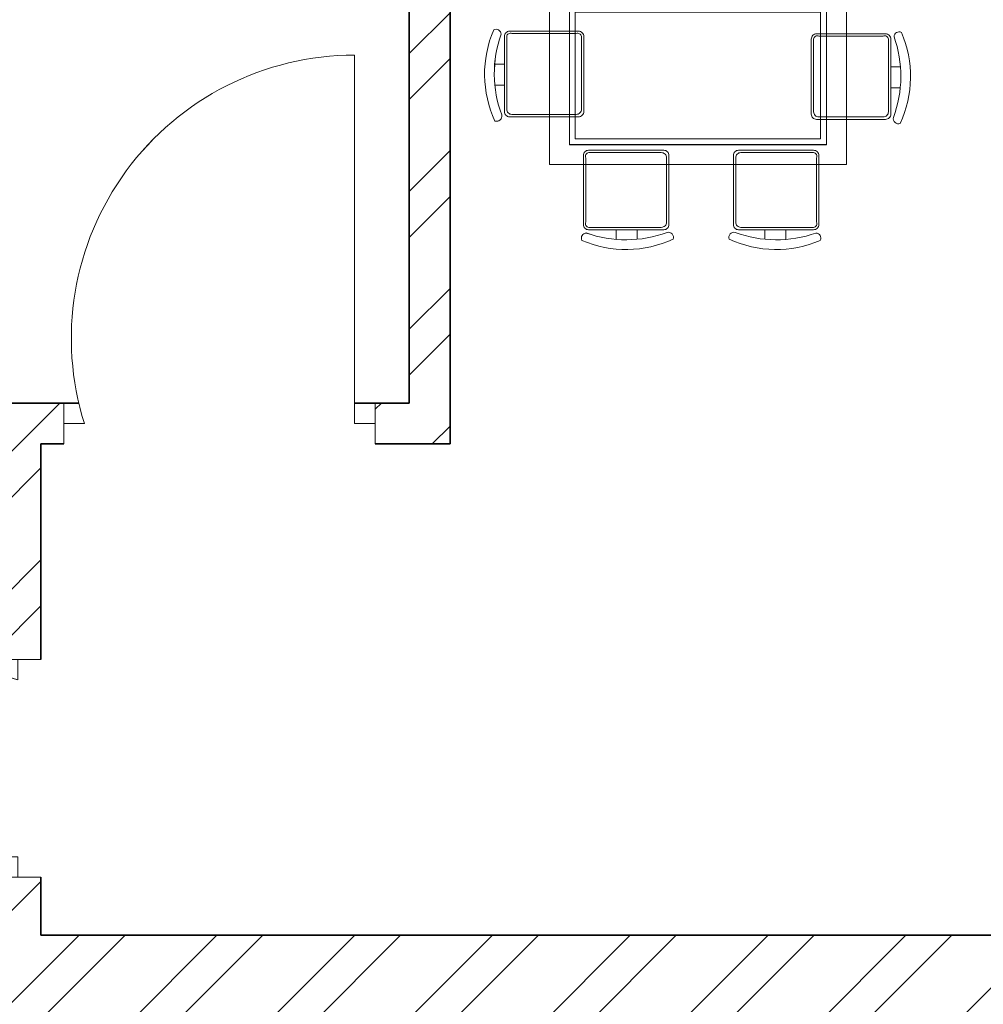
# Model space of a CAD drawing. Units: inches. Extents: x 2120 to 4013, y 1390 to 3019.
# Tile 8 of 59: x 2354 to 2448, y 1868 to 1964. Entities that reach past the tile are written whole.
import ezdxf

# ---------------------------------------------------------------- set-up
doc = ezdxf.new("R2010")
doc.units = ezdxf.units.IN
for name, color, linetype, lineweight in [('A-DOOR', 3, 'Continuous', 18), ('A-FURN', 8, 'Continuous', 13), ('A-WALL', 7, 'Continuous', 35), ('A-WALL-PATT', 252, 'Continuous', 13)]:
    doc.layers.add(name, color=color, linetype=linetype, lineweight=lineweight)

# ---------------------------------------------------------------- blocks, each defined once
blk = doc.blocks.new('DOOR-SWING-24IN-108p49DEG')
for p, q in [((21.75, 21.28), (26.25, 21.28)), ((26.25, 21.28), (24, 21.28)), ((24, 21.28), (24, 19.28)), ((24, 2), (0, 2)), ((24, 0), (24, 2)), ((26.25, 0), (21.75, 0)), ((21.75, 0), (24, 0))]:
    blk.add_line(p, q)
blk.add_arc((18.221, 2), 18.221, 71.50887, 180)
blk = doc.blocks.new('DOOR-SWING-36IN-107p46DEG')
for p, q in [((28.418, 2), (28.418, 38)), ((0, 0), (0, 4)), ((0, 4), (0, 2)), ((30.418, 4), (30.418, 0)), ((0, 2), (2, 2)), ((30.418, 2), (28.418, 2)), ((30.418, 0), (30.418, 2))]:
    blk.add_line(p, q)
blk.add_arc((28.418, 10.307), 27.693, 90, 197.45547)
blk = doc.blocks.new('TABLE-DINING')
for points in [[(0, 17.406), (29.011, 17.406), (29.011, 0), (0, 0)], [(1.934, 15.472), (27.077, 15.472), (27.077, 1.934), (1.934, 1.934)], [(2.514, 14.892), (26.496, 14.892), (26.496, 2.514), (2.514, 2.514)]]:
    blk.add_lwpolyline(points, close=True)
blk = doc.blocks.new('CHAIR-DINING-04')
for points in [[(7.771, 8.294, 0.414214), (7.258, 8.807), (0.513, 8.807, 0.414214), (0, 8.294), (0, 0.958, 0.414214), (0.513, 0.445), (7.258, 0.445, 0.414214), (7.771, 0.958), (7.771, 8.294)], [(8.089, 8.525, -0.175809), (8.029, 0.623, 0.578392), (8.687, 0.025, 0.214524), (8.807, 8.944, 0.552014), (8.089, 8.525, -0.065079)], [(7.771, 3.535), (8.699, 3.535, -0.064759)]]:
    blk.add_lwpolyline(points, format="xyb")
blk.add_lwpolyline([(7.54, 8.291), (7.54, 1.19, -0.414214), (7.027, 0.676), (0.744, 0.676, -0.414214), (0.231, 1.19), (0.231, 8.291, -0.512069), (0.744, 8.576), (7.027, 8.576, -0.512069)], format="xyb", close=True)
blk.add_lwpolyline([(8.716, 5.588), (7.771, 5.588)])
blk = doc.blocks.new('CHAIR-DINING-05')
for points in [[(1.676, 0.623, -0.578392), (1.018, 0.025, -0.214524), (0.898, 8.944, -0.552014), (1.616, 8.525, 0.175809), (1.676, 0.623)], [(1.933, 8.294, -0.414214), (2.446, 8.807), (9.191, 8.807, -0.414214), (9.704, 8.294), (9.704, 0.958, -0.414214), (9.191, 0.445), (2.446, 0.445, -0.414214), (1.933, 0.958), (1.933, 8.294)], [(1.933, 3.535), (1.005, 3.535, 0.064759)]]:
    blk.add_lwpolyline(points, format="xyb")
blk.add_lwpolyline([(2.164, 8.291), (2.164, 1.19, 0.414214), (2.677, 0.676), (8.96, 0.676, 0.414214), (9.473, 1.19), (9.473, 8.291, 0.512069), (8.96, 8.576), (2.677, 8.576, 0.512069)], format="xyb", close=True)
blk.add_lwpolyline([(0.988, 5.588), (1.933, 5.588)])
blk = doc.blocks.new('CHAIR-DINING-10')
for points in [[(0.623, 8.029, -0.578392), (0.025, 8.687, -0.214524), (8.944, 8.807, -0.552014), (8.525, 8.089, 0.175809), (0.623, 8.029)], [(3.535, 7.771), (3.535, 8.699, 0.064759)], [(8.294, 7.771, -0.414214), (8.807, 7.258), (8.807, 0.513, -0.414214), (8.294, 0), (0.958, 0, -0.414214), (0.445, 0.513), (0.445, 7.258, -0.414214), (0.958, 7.771), (8.294, 7.771)]]:
    blk.add_lwpolyline(points, format="xyb")
blk.add_lwpolyline([(5.588, 8.716), (5.588, 7.771)])
blk.add_lwpolyline([(8.291, 7.54), (1.19, 7.54, 0.414214), (0.676, 7.027), (0.676, 0.744, 0.414214), (1.19, 0.231), (8.291, 0.231, 0.512069), (8.576, 0.744), (8.576, 7.027, 0.512069)], format="xyb", close=True)
blk = doc.blocks.new('CHAIR-DINING-15')
for points in [[(8.294, 1.933, 0.414214), (8.807, 2.446), (8.807, 9.191, 0.414214), (8.294, 9.704), (0.958, 9.704, 0.414214), (0.445, 9.191), (0.445, 2.446, 0.414214), (0.958, 1.933), (8.294, 1.933)], [(3.535, 1.933), (3.535, 1.005, -0.064759)], [(8.525, 1.616, -0.175809), (0.623, 1.676, 0.578392), (0.025, 1.018, 0.214524), (8.944, 0.898, 0.552014), (8.525, 1.616, -0.065079)]]:
    blk.add_lwpolyline(points, format="xyb")
blk.add_lwpolyline([(8.291, 2.164), (1.19, 2.164, -0.414214), (0.676, 2.677), (0.676, 8.96, -0.414214), (1.19, 9.473), (8.291, 9.473, -0.512069), (8.576, 8.96), (8.576, 2.677, -0.512069)], format="xyb", close=True)
blk.add_lwpolyline([(5.588, 0.988), (5.588, 1.933)])

msp = doc.modelspace()

# ---------------------------------------------------------------- hatches: boundary and pattern name
at = {"layer": 'A-WALL-PATT'}
h = msp.add_hatch(dxfattribs=at)
h.set_pattern_fill('ANSI32', color=256)
h.paths.add_polyline_path([(2271.7331, 1980.389), (2262.7331, 1980.389), (2262.7331, 1912.8434), (2267.2331, 1912.8434), (2271.7331, 1912.8434), (2271.7331, 1922.531), (2351.2331, 1922.531), (2351.2331, 1901.4728), (2355.7331, 1901.4728), (2355.7331, 1922.531), (2357.9815, 1922.531), (2357.9815, 1926.5306), (2271.7331, 1926.5306)])
h.paths.add_polyline_path([(2589.2331, 1949.1622), (2584.7331, 1949.1622), (2580.2331, 1949.1622), (2580.2331, 1874.5306), (2355.7331, 1874.5306), (2355.7331, 1880.1922), (2351.2331, 1880.1922), (2351.2331, 1874.5306), (2271.7331, 1874.5306), (2271.7331, 1888.8431), (2262.7331, 1888.8431), (2262.7331, 1842.2909), (2267.2331, 1842.2909), (2271.7331, 1842.2909), (2271.7331, 1865.531), (2415.7331, 1865.531), (2415.7331, 1779.7286), (2420.2331, 1779.7286), (2420.2331, 1865.531), (2589.2331, 1865.531)])
h.paths.add_polyline_path([(2271.7331, 1782.2906), (2262.7331, 1782.2906), (2262.7331, 1711.4639), (2267.2331, 1711.4639), (2271.7331, 1711.4639), (2271.7331, 1738.031), (2420.2331, 1738.031), (2420.2331, 1742.531), (2420.2331, 1747.3376), (2417.9831, 1747.3376), (2415.7331, 1747.3376), (2415.7331, 1742.5306), (2271.7331, 1742.5306)])
h.paths.add_polyline_path([(2271.7331, 1627.031), (2362.3957, 1627.031), (2362.3957, 1629.281), (2362.3957, 1631.5306), (2271.7331, 1631.5306), (2271.7331, 1675.4636), (2262.7331, 1675.4636), (2262.7331, 1581.531), (2405.3032, 1581.531), (2405.3032, 1586.031), (2405.3032, 1590.5306), (2396.2331, 1590.5306), (2396.2331, 1691.4513), (2418.7206, 1691.4513), (2418.7206, 1695.951), (2396.2331, 1695.951), (2391.7331, 1695.951), (2391.7331, 1631.5306), (2386.7425, 1631.5306), (2386.7425, 1629.2806), (2386.7425, 1627.031), (2391.7331, 1627.031), (2391.7331, 1586.1709), (2271.7331, 1586.1709)])
h.paths.add_polyline_path([(2459.6703, 1590.5306), (2429.3032, 1590.5306), (2429.3032, 1581.531), (2459.6703, 1581.531), (2459.6703, 1586.031)])
h.paths.add_polyline_path([(2501.2331, 1590.531), (2501.2331, 1665.0195), (2498.9831, 1665.0195), (2496.7331, 1665.0195), (2496.7331, 1590.5306), (2483.8201, 1590.5306), (2483.8201, 1590.1579), (2483.6704, 1590.1579), (2483.6704, 1581.531), (2505.0196, 1581.531), (2505.0196, 1583.781), (2505.0196, 1586.0306), (2501.2331, 1586.0306)])
h.paths.add_polyline_path([(2544.1361, 1583.781), (2544.1361, 1586.0306), (2527.1368, 1586.0306), (2527.1368, 1583.7806), (2527.1368, 1581.531), (2544.1361, 1581.531)])
h.paths.add_polyline_path([(3822.6535, 2458.4402), (3874.9468, 2458.4402), (3874.9468, 2476.9866), (3822.6535, 2476.9866)], flags=9)
h.paths.add_polyline_path([(3834.6921, 2781.8174), (3935.9206, 2781.8174), (3935.9206, 2800.3638), (3834.6921, 2800.3638)], flags=9)
h.paths.add_polyline_path([(3832.2843, 2837.9683), (3884.5776, 2837.9683), (3884.5776, 2856.5146), (3832.2843, 2856.5146)], flags=9)
h.paths.add_polyline_path([(3830.9388, 2861.4782), (3956.8958, 2861.4782), (3956.8958, 2880.0245), (3830.9388, 2880.0245)], flags=9)
h.paths.add_polyline_path([(3870.6966, 2352.5752), (3887.9272, 2352.5752), (3887.9272, 2377.3037), (3870.6966, 2377.3037)], flags=9)
h.paths.add_polyline_path([(3289.2701, 2413.161), (3435.2223, 2413.161), (3435.2223, 2450.2538), (3289.2701, 2450.2538)], flags=9)
h.paths.add_polyline_path([(2487.6944, 2414.3601), (2637.8335, 2414.3601), (2637.8335, 2451.4528), (2487.6944, 2451.4528)], flags=9)
h.paths.add_polyline_path([(2567.3724, 1457.9199), (2815.296, 1457.9199), (2815.296, 1495.0127), (2567.3724, 1495.0127)], flags=9)
h.paths.add_polyline_path([(2655.3825, 2093.2363), (2685.9555, 2093.2363), (2685.9555, 2111.8937), (2655.3825, 2111.8937)], flags=9)
h.paths.add_polyline_path([(2543.9218, 1550.6671), (2587.8406, 1550.6671), (2587.8406, 1569.3244), (2543.9218, 1569.3244)], flags=9)
h.paths.add_polyline_path([(2905.1384, 1543.8113), (2949.0572, 1543.8113), (2949.0572, 1562.4686), (2905.1384, 1562.4686)], flags=9)
h.paths.add_polyline_path([(2736.4118, 1702.4736), (2784.2153, 1702.4736), (2784.2153, 1721.1309), (2736.4118, 1721.1309)], flags=9)
h.paths.add_polyline_path([(2912.8666, 1710.4168), (2951.707, 1710.4168), (2951.707, 1729.0741), (2912.8666, 1729.0741)], flags=9)
h.paths.add_polyline_path([(2923.5785, 1763.5038), (2959.7279, 1763.5038), (2959.7279, 1782.1611), (2923.5785, 1782.1611)], flags=9)
h.paths.add_polyline_path([(2925.2114, 1809.6137), (2967.1861, 1809.6137), (2967.1861, 1828.271), (2925.2114, 1828.271)], flags=9)
h.paths.add_polyline_path([(2996.2711, 1878.9003), (2996.2711, 1913.109), (2977.6138, 1913.109), (2977.6138, 1878.9003)], flags=9)
h.paths.add_polyline_path([(2883.0859, 1895.7192), (2927.1855, 1895.7192), (2927.1855, 1914.3766), (2883.0859, 1914.3766)], flags=9)
h.paths.add_polyline_path([(2787.3924, 1810.8013), (2841.0213, 1810.8013), (2841.0213, 1829.4587), (2787.3924, 1829.4587)], flags=9)
h.paths.add_polyline_path([(2775.6399, 2101.7395), (2829.2689, 2101.7395), (2829.2689, 2120.3968), (2775.6399, 2120.3968)], flags=9)
h.paths.add_polyline_path([(2913.0263, 2075.817), (2951.8667, 2075.817), (2951.8667, 2094.4744), (2913.0263, 2094.4744)], flags=9)
h.paths.add_polyline_path([(2929.966, 2133.3669), (2966.1154, 2133.3669), (2966.1154, 2152.0243), (2929.966, 2152.0243)], flags=9)
h.paths.add_polyline_path([(2932.7502, 2182.6088), (2968.8996, 2182.6088), (2968.8996, 2201.2662), (2932.7502, 2201.2662)], flags=9)
h.paths.add_polyline_path([(2996.0681, 2266.3173), (2996.0681, 2300.5261), (2977.4108, 2300.5261), (2977.4108, 2266.3173)], flags=9)
h.paths.add_polyline_path([(2885.1039, 2279.2186), (2929.2035, 2279.2186), (2929.2035, 2297.8759), (2885.1039, 2297.8759)], flags=9)
h.paths.add_polyline_path([(2735.7042, 2218.3197), (2783.5078, 2218.3197), (2783.5078, 2236.9771), (2735.7042, 2236.9771)], flags=9)
h.paths.add_polyline_path([(2635.6049, 2044.0085), (2648.9678, 2044.0085), (2648.9678, 2054.312), (2635.6049, 2054.312)], flags=9)
h.paths.add_polyline_path([(2714.0148, 1923.0473), (2727.3777, 1923.0473), (2727.3777, 1933.3508), (2714.0148, 1933.3508)], flags=9)
h.paths.add_polyline_path([(2709.0345, 1988.1628), (2722.3974, 1988.1628), (2722.3974, 1998.4663), (2709.0345, 1998.4663)], flags=9)
h.paths.add_polyline_path([(2592.8935, 1962.1763), (2606.2564, 1962.1763), (2606.2564, 1972.4799), (2592.8935, 1972.4799)], flags=9)
h.paths.add_polyline_path([(2618.3996, 1985.9724), (2644.1942, 1985.9724), (2644.1942, 1996.2759), (2618.3996, 1996.2759)], flags=9)
h.paths.add_polyline_path([(2601.279, 1920.5869), (2614.6419, 1920.5869), (2614.6419, 1930.8904), (2601.279, 1930.8904)], flags=9)
h.paths.add_polyline_path([(2692.3278, 1932.7645), (2704.5311, 1932.7645), (2704.5311, 1943.0681), (2692.3278, 1943.0681)], flags=9)
h.paths.add_polyline_path([(2311.122, 1672.7318), (2355.0408, 1672.7318), (2355.0408, 1691.3892), (2311.122, 1691.3892)], flags=25)
h.paths.add_polyline_path([(2456.2551, 1632.3198), (2492.4796, 1632.3198), (2492.4796, 1650.9772), (2456.2551, 1650.9772)], flags=9)
h.paths.add_polyline_path([(2401.0766, 1631.4793), (2437.301, 1631.4793), (2437.301, 1650.1367), (2401.0766, 1650.1367)], flags=9)
h.paths.add_polyline_path([(2546.7054, 1700.9235), (2594.509, 1700.9235), (2594.509, 1719.5809), (2546.7054, 1719.5809)], flags=9)
h.paths.add_polyline_path([(2445.4866, 1766.9937), (2497.5261, 1766.9937), (2497.5261, 1785.651), (2445.4866, 1785.651)], flags=9)
h.paths.add_polyline_path([(2287.9992, 1739.7675), (2326.8396, 1739.7675), (2326.8396, 1758.4248), (2287.9992, 1758.4248)], flags=24)
h.paths.add_polyline_path([(2458.5279, 1924.7607), (2510.5675, 1924.7607), (2510.5675, 1943.4181), (2458.5279, 1943.4181)], flags=25)
h.paths.add_polyline_path([(2309.2811, 1902.7642), (2345.4305, 1902.7642), (2345.4305, 1921.4215), (2309.2811, 1921.4215)], flags=25)
h.paths.add_polyline_path([(2490.7554, 2018.9392), (2530.7896, 2018.9392), (2530.7896, 2037.5965), (2490.7554, 2037.5965)], flags=9)
h.paths.add_polyline_path([(2402.143, 2024.7393), (2438.5414, 2024.7393), (2438.5414, 2043.3966), (2402.143, 2043.3966)], flags=9)
h.paths.add_polyline_path([(2287.856, 1931.7926), (2326.6964, 1931.7926), (2326.6964, 1950.4499), (2287.856, 1950.4499)], flags=25)
h.paths.add_polyline_path([(2281.7979, 2193.5771), (2320.6383, 2193.5771), (2320.6383, 2212.2344), (2281.7979, 2212.2344)], flags=9)
h.paths.add_polyline_path([(2484.0754, 2093.892), (2536.115, 2093.892), (2536.115, 2112.5494), (2484.0754, 2112.5494)], flags=9)
h.paths.add_polyline_path([(2624.7948, 2281.8639), (2624.7948, 2311.4137), (2606.1375, 2311.4137), (2606.1375, 2281.8639)], flags=9)
h.paths.add_polyline_path([(2507.5036, 2290.3639), (2541.934, 2290.3639), (2541.934, 2309.0212), (2507.5036, 2309.0212)], flags=9)
h.paths.add_polyline_path([(2423.1076, 2285.2202), (2459.332, 2285.2202), (2459.332, 2303.8776), (2423.1076, 2303.8776)], flags=9)
h.paths.add_polyline_path([(2374.5467, 2289.6272), (2410.7711, 2289.6272), (2410.7711, 2308.2846), (2374.5467, 2308.2846)], flags=9)
h.paths.add_polyline_path([(2277.4907, 2227.5651), (2316.3311, 2227.5651), (2316.3311, 2246.2224), (2277.4907, 2246.2224)], flags=9)
h.paths.add_polyline_path([(2655.3825, 2093.2367), (2685.9555, 2093.2367), (2685.9555, 2111.894), (2655.3825, 2111.894)], flags=9)
h.paths.add_polyline_path([(2543.9217, 1550.6674), (2587.8406, 1550.6674), (2587.8406, 1569.3247), (2543.9217, 1569.3247)], flags=9)
h.paths.add_polyline_path([(2905.1384, 1543.8116), (2949.0572, 1543.8116), (2949.0572, 1562.4689), (2905.1384, 1562.4689)], flags=9)
h.paths.add_polyline_path([(2736.4118, 1702.4739), (2784.2153, 1702.4739), (2784.2153, 1721.1312), (2736.4118, 1721.1312)], flags=9)
h.paths.add_polyline_path([(2912.8666, 1710.4171), (2951.707, 1710.4171), (2951.707, 1729.0744), (2912.8666, 1729.0744)], flags=9)
h.paths.add_polyline_path([(2923.5785, 1763.5041), (2959.7279, 1763.5041), (2959.7279, 1782.1614), (2923.5785, 1782.1614)], flags=9)
h.paths.add_polyline_path([(2925.2114, 1809.614), (2967.1861, 1809.614), (2967.1861, 1828.2713), (2925.2114, 1828.2713)], flags=9)
h.paths.add_polyline_path([(2996.2711, 1878.9006), (2996.2711, 1913.1094), (2977.6137, 1913.1094), (2977.6137, 1878.9006)], flags=9)
h.paths.add_polyline_path([(2883.0859, 1895.7195), (2927.1855, 1895.7195), (2927.1855, 1914.3769), (2883.0859, 1914.3769)], flags=9)
h.paths.add_polyline_path([(2787.3924, 1810.8016), (2841.0213, 1810.8016), (2841.0213, 1829.459), (2787.3924, 1829.459)], flags=9)
h.paths.add_polyline_path([(2775.6399, 2101.7398), (2829.2688, 2101.7398), (2829.2688, 2120.3971), (2775.6399, 2120.3971)], flags=9)
h.paths.add_polyline_path([(2913.0263, 2075.8173), (2951.8667, 2075.8173), (2951.8667, 2094.4747), (2913.0263, 2094.4747)], flags=9)
h.paths.add_polyline_path([(2929.966, 2133.3672), (2966.1154, 2133.3672), (2966.1154, 2152.0246), (2929.966, 2152.0246)], flags=9)
h.paths.add_polyline_path([(2932.7502, 2182.6091), (2968.8996, 2182.6091), (2968.8996, 2201.2665), (2932.7502, 2201.2665)], flags=9)
h.paths.add_polyline_path([(2996.0681, 2266.3176), (2996.0681, 2300.5264), (2977.4108, 2300.5264), (2977.4108, 2266.3176)], flags=9)
h.paths.add_polyline_path([(2885.1039, 2279.2189), (2929.2035, 2279.2189), (2929.2035, 2297.8762), (2885.1039, 2297.8762)], flags=9)
h.paths.add_polyline_path([(2735.7042, 2218.32), (2783.5078, 2218.32), (2783.5078, 2236.9774), (2735.7042, 2236.9774)], flags=9)
h.paths.add_polyline_path([(2635.6048, 2044.0088), (2648.9677, 2044.0088), (2648.9677, 2054.3123), (2635.6048, 2054.3123)], flags=9)
h.paths.add_polyline_path([(2714.0148, 1923.0476), (2727.3777, 1923.0476), (2727.3777, 1933.3511), (2714.0148, 1933.3511)], flags=9)
h.paths.add_polyline_path([(2709.0345, 1988.1631), (2722.3974, 1988.1631), (2722.3974, 1998.4666), (2709.0345, 1998.4666)], flags=9)
h.paths.add_polyline_path([(2592.8935, 1962.1766), (2606.2564, 1962.1766), (2606.2564, 1972.4802), (2592.8935, 1972.4802)], flags=9)
h.paths.add_polyline_path([(2618.3995, 1985.9727), (2644.1942, 1985.9727), (2644.1942, 1996.2762), (2618.3995, 1996.2762)], flags=9)
h.paths.add_polyline_path([(2601.279, 1920.5872), (2614.6419, 1920.5872), (2614.6419, 1930.8908), (2601.279, 1930.8908)], flags=9)
h.paths.add_polyline_path([(2692.3278, 1932.7648), (2704.5311, 1932.7648), (2704.5311, 1943.0684), (2692.3278, 1943.0684)], flags=9)
h.paths.add_polyline_path([(2311.122, 1672.7321), (2355.0408, 1672.7321), (2355.0408, 1691.3895), (2311.122, 1691.3895)], flags=25)
h.paths.add_polyline_path([(2456.2551, 1632.3201), (2492.4795, 1632.3201), (2492.4795, 1650.9775), (2456.2551, 1650.9775)], flags=9)
h.paths.add_polyline_path([(2401.0766, 1631.4796), (2437.301, 1631.4796), (2437.301, 1650.137), (2401.0766, 1650.137)], flags=9)
h.paths.add_polyline_path([(2546.7054, 1700.9238), (2594.509, 1700.9238), (2594.509, 1719.5812), (2546.7054, 1719.5812)], flags=9)
h.paths.add_polyline_path([(2445.4866, 1766.994), (2497.5261, 1766.994), (2497.5261, 1785.6513), (2445.4866, 1785.6513)], flags=9)
h.paths.add_polyline_path([(2287.9992, 1739.7678), (2326.8396, 1739.7678), (2326.8396, 1758.4251), (2287.9992, 1758.4251)], flags=24)
h.paths.add_polyline_path([(2458.5279, 1924.7611), (2510.5675, 1924.7611), (2510.5675, 1943.4184), (2458.5279, 1943.4184)], flags=25)
h.paths.add_polyline_path([(2309.2811, 1902.7645), (2345.4305, 1902.7645), (2345.4305, 1921.4218), (2309.2811, 1921.4218)], flags=25)
h.paths.add_polyline_path([(2490.7554, 2018.9395), (2530.7895, 2018.9395), (2530.7895, 2037.5968), (2490.7554, 2037.5968)], flags=9)
h.paths.add_polyline_path([(2402.143, 2024.7396), (2438.5413, 2024.7396), (2438.5413, 2043.3969), (2402.143, 2043.3969)], flags=9)
h.paths.add_polyline_path([(2287.856, 1931.7929), (2326.6964, 1931.7929), (2326.6964, 1950.4502), (2287.856, 1950.4502)], flags=25)
h.paths.add_polyline_path([(2281.7979, 2193.5774), (2320.6383, 2193.5774), (2320.6383, 2212.2347), (2281.7979, 2212.2347)], flags=9)
h.paths.add_polyline_path([(2484.0754, 2093.8924), (2536.115, 2093.8924), (2536.115, 2112.5497), (2484.0754, 2112.5497)], flags=9)
h.paths.add_polyline_path([(2624.7948, 2281.8642), (2624.7948, 2311.414), (2606.1374, 2311.414), (2606.1374, 2281.8642)], flags=9)
h.paths.add_polyline_path([(2507.5035, 2290.3642), (2541.934, 2290.3642), (2541.934, 2309.0215), (2507.5035, 2309.0215)], flags=9)
h.paths.add_polyline_path([(2423.1075, 2285.2205), (2459.332, 2285.2205), (2459.332, 2303.8779), (2423.1075, 2303.8779)], flags=9)
h.paths.add_polyline_path([(2374.5467, 2289.6275), (2410.7711, 2289.6275), (2410.7711, 2308.2849), (2374.5467, 2308.2849)], flags=9)
h.paths.add_polyline_path([(2277.4907, 2227.5654), (2316.3311, 2227.5654), (2316.3311, 2246.2227), (2277.4907, 2246.2227)], flags=9)
h = msp.add_hatch(dxfattribs=at)
h.set_pattern_fill('ANSI32', color=256)
h.paths.add_polyline_path([(2271.7331, 2122.6377), (2262.7331, 2122.6377), (2262.7331, 2040.3893), (2267.2331, 2040.3893), (2271.7331, 2040.3893), (2271.7331, 2044.8856), (2271.7331, 2070.531), (2391.7331, 2070.531), (2391.7331, 1926.5306), (2388.3993, 1926.5306), (2388.3993, 1922.531), (2395.7331, 1922.531), (2395.7331, 1992.531), (2400.4511, 1992.531), (2400.4511, 1997.0306), (2395.7331, 1997.0306), (2395.7331, 2070.531), (2443.7331, 2070.531), (2443.7331, 2046.1368), (2448.2331, 2046.1368), (2448.2331, 2070.531), (2580.2331, 2070.531), (2580.2331, 1997.0306), (2492.9076, 1997.0306), (2492.9076, 1992.531), (2580.2331, 1992.531), (2580.2331, 1983.9368), (2589.2331, 1983.9368), (2589.2331, 2070.531), (2589.2331, 2075.0306), (2396.2331, 2075.0306), (2396.2331, 2184.3565), (2393.9831, 2184.3565), (2391.7331, 2184.3565), (2391.7331, 2075.0306), (2271.7331, 2075.0306)])
h.paths.add_polyline_path([(2724.7331, 2138.0306), (2628.7331, 2138.0306), (2628.7331, 2070.5306), (2628.7331, 2067.0987), (2633.2331, 2067.0987), (2637.7331, 2067.0987), (2637.7331, 2070.531), (2657.3413, 2070.531), (2657.3413, 2079.5306), (2637.7331, 2079.5306), (2637.7331, 2129.031), (2715.7331, 2129.031), (2715.7331, 2079.5306), (2698.0378, 2079.5306), (2698.0378, 2070.531), (2715.7331, 2070.531), (2715.7331, 2012.1531), (2720.2331, 2012.1531), (2724.7331, 2012.1531)])
h.paths.add_polyline_path([(2724.7331, 2213.031), (2831.3209, 2213.031), (2831.3209, 2215.281), (2831.3209, 2217.5306), (2724.7331, 2217.5306), (2724.7331, 2343.531), (2751.8755, 2343.531), (2751.8755, 2352.5306), (2715.7331, 2352.5306), (2715.7331, 2138.031), (2724.7331, 2138.031)])
h.paths.add_polyline_path([(2902.53, 2352.5306), (2811.8755, 2352.5306), (2811.8755, 2343.531), (2867.2331, 2343.531), (2867.2331, 2217.5306), (2863.6364, 2217.5306), (2863.6364, 2213.031), (2871.7331, 2213.031), (2871.7331, 2217.531), (2871.7331, 2343.531), (2902.53, 2343.531)])
h.paths.add_polyline_path([(3009.7331, 2352.5306), (2938.53, 2352.5306), (2938.53, 2343.531), (2966.2331, 2343.531), (2966.2331, 2242.3281), (2968.4831, 2242.3281), (2970.7331, 2242.3281), (2970.7331, 2343.531), (3009.7331, 2343.531)])
h.paths.add_polyline_path([(3009.7331, 2217.5306), (2970.7331, 2217.5306), (2970.7331, 2220.5422), (2968.4831, 2220.5422), (2966.2331, 2220.5422), (2966.2331, 2217.5306), (2911.7752, 2217.5306), (2907.7331, 2217.5306), (2907.7331, 2213.0306), (2907.7331, 2194.9663), (2912.2331, 2194.9663), (2912.2331, 2213.031), (2970.7331, 2213.031), (3000.7331, 2213.031), (3000.7331, 2205.523), (3009.7331, 2205.523)])
h.paths.add_polyline_path([(3009.7331, 2181.5227), (3000.7331, 2181.5227), (3000.7331, 2165.0306), (2912.2331, 2165.0306), (2912.2331, 2170.8202), (2907.7331, 2170.8202), (2907.7331, 2165.0306), (2899.5169, 2165.0306), (2899.5169, 2162.7806), (2899.5169, 2160.531), (2907.7331, 2160.531), (2907.7331, 2137.3432), (2912.2331, 2137.3432), (2912.2331, 2160.531), (3000.7331, 2160.531), (3000.7331, 2150.4993), (3009.7331, 2150.4993)])
h.paths.add_polyline_path([(3009.7331, 2126.499), (3005.2331, 2126.499), (3000.7331, 2126.499), (3000.7331, 2112.5306), (2912.2331, 2112.5306), (2912.2331, 2115.6036), (2907.7331, 2115.6036), (2907.7331, 2108.031), (3000.7331, 2108.031), (3000.7331, 2084.7256), (3009.7331, 2084.7256)], flags=17)
h.paths.add_polyline_path([(3009.7331, 1971.531), (3009.7331, 2024.7253), (3000.7331, 2024.7253), (3000.7331, 2006.4153), (3000.7331, 1971.5306), (2864.2331, 1971.5306), (2864.2331, 2160.531), (2868.0522, 2160.531), (2868.0522, 2165.0306), (2859.7331, 2165.0306), (2859.7331, 1971.5306), (2724.7331, 1971.5306), (2724.7331, 1977.7012), (2715.7331, 1977.7012), (2715.7331, 1962.5306), (2715.7331, 1950.9035), (2720.2331, 1950.9035), (2724.7331, 1950.9035), (2724.7331, 1962.531), (2855.2331, 1962.531), (2859.7331, 1962.531), (2859.7331, 1835.031), (2864.2331, 1834.8158), (2864.2331, 1962.531), (2958.7331, 1962.531), (2958.7331, 1937.0925), (2963.2331, 1937.0925), (2963.2331, 1962.531), (3000.7331, 1962.531), (3009.7331, 1962.531)])
h.paths.add_polyline_path([(2724.7331, 1728.531), (2822.7164, 1728.531), (2822.7164, 1733.0306), (2724.7331, 1733.0306), (2724.7331, 1779.3416), (2715.7331, 1779.3416), (2715.7331, 1581.531), (2753.02, 1581.531), (2753.02, 1586.031), (2753.02, 1590.5306), (2724.7331, 1590.5306)])
h.paths.add_polyline_path([(2864.2331, 1590.531), (2864.2331, 1787.031), (2868.4075, 1787.031), (2868.4075, 1791.5306), (2859.7331, 1791.5306), (2859.7331, 1739.0306), (2859.7331, 1733.0306), (2854.3125, 1733.0306), (2854.3125, 1728.531), (2859.7331, 1728.531), (2859.7331, 1590.5306), (2813.02, 1590.5306), (2813.02, 1581.531), (2868.4123, 1581.531), (2868.4123, 1583.781), (2868.4123, 1586.0306), (2864.2331, 1586.0306)])
h.paths.add_polyline_path([(3009.7331, 1754.6619), (3000.7331, 1754.6619), (3000.7331, 1739.0306), (2912.2331, 1739.0306), (2912.2331, 1742.2257), (2907.7331, 1742.2257), (2907.7331, 1739.0306), (2907.7331, 1734.531), (3000.7331, 1734.531), (3000.7331, 1590.5306), (3000.7331, 1586.0306), (2971.3921, 1586.0306), (2971.3921, 1581.531), (3009.7331, 1581.531)])
h.paths.add_polyline_path([(2911.3921, 1583.781), (2911.3921, 1586.0306), (2891.2138, 1586.0306), (2891.2138, 1581.531), (2911.3921, 1581.531)])
h.paths.add_polyline_path([(3009.7331, 1799.8422), (3000.7331, 1799.8422), (3000.7331, 1791.5306), (2912.2331, 1791.5306), (2912.2331, 1796.3264), (2909.9831, 1796.3264), (2907.7331, 1796.3264), (2907.7331, 1791.5306), (2902.7033, 1791.5306), (2902.7033, 1787.031), (2907.7331, 1787.031), (2907.7331, 1761.1622), (2912.2331, 1761.1622), (2912.2331, 1787.031), (3000.7331, 1787.031), (3000.7331, 1778.6622), (3009.7331, 1778.6622)])
h.paths.add_polyline_path([(3009.7331, 1839.5306), (2963.2331, 1839.5306), (2963.2331, 1842.8629), (2960.9831, 1842.8629), (2958.7331, 1842.8629), (2958.7331, 1839.5306), (2907.7331, 1839.5306), (2907.7331, 1814.4599), (2912.2331, 1814.4599), (2912.2331, 1835.031), (3000.7331, 1835.031), (3000.7331, 1823.8425), (3009.7331, 1823.8425), (3009.7331, 1835.031)])
h.paths.add_polyline_path([(2963.2331, 1901.0922), (2960.9831, 1901.0922), (2958.7331, 1901.0922), (2958.7331, 1862.8843), (2963.2331, 1862.8843)], flags=17)
h.paths.add_polyline_path([(2724.7331, 1891.9826), (2724.7331, 1914.3416), (2715.7331, 1914.3416), (2715.7331, 1783.8416), (2637.7331, 1783.8416), (2637.7331, 1914.3416), (2628.7331, 1914.3416), (2624.7701, 1914.3416), (2624.7701, 1909.8416), (2624.7701, 1905.3419), (2628.7331, 1905.3419), (2628.7331, 1876.9915), (2628.7331, 1779.3419), (2637.7331, 1779.3419), (2715.7331, 1779.3419), (2724.7331, 1779.3419), (2724.7331, 1835.031)])
h.paths.add_polyline_path([(2637.7331, 1731.531), (2637.7331, 1779.3416), (2628.7331, 1779.3416), (2628.7331, 1731.5306), (2589.2331, 1731.5306), (2535.9814, 1731.5306), (2496.7331, 1731.5306), (2496.7331, 1725.6876), (2498.9831, 1725.6876), (2501.2331, 1725.6876), (2501.2331, 1727.031), (2628.7331, 1727.031), (2628.7331, 1680.4203), (2628.7331, 1590.5306), (2628.7331, 1586.0306), (2604.1361, 1586.0306), (2604.1361, 1581.531), (2637.7331, 1581.531), (2637.7331, 1590.531)])

# ---------------------------------------------------------------- linework, layer by layer
at = {"layer": 'A-FURN'}
for points in [[(2438.8103, 1962.1042, 0.4142136), (2438.2971, 1962.6174), (2431.5521, 1962.6174, 0.4142136), (2431.0389, 1962.1042), (2431.0389, 1954.7686, 0.4142136), (2431.5521, 1954.2553), (2438.2971, 1954.2553, 0.4142136), (2438.8103, 1954.7686), (2438.8103, 1962.1042)], [(2438.8104, 1962.1039, 0.4142136), (2438.2971, 1962.6171), (2431.5521, 1962.6171, 0.4142136), (2431.0389, 1962.1039), (2431.0389, 1954.7683, 0.4142136), (2431.5521, 1954.255), (2438.2971, 1954.255, 0.4142136), (2438.8104, 1954.7683), (2438.8104, 1962.1039)], [(2439.1275, 1962.335, -0.1758092), (2439.0676, 1954.4333, 0.5783921), (2439.7259, 1953.8347, 0.2145244), (2439.8455, 1962.7541, 0.552014), (2439.1275, 1962.335, -0.065079)], [(2439.1275, 1962.3347, -0.1758092), (2439.0677, 1954.433, 0.5783921), (2439.7259, 1953.8344, 0.2145244), (2439.8456, 1962.7538, 0.552014), (2439.1275, 1962.3347, -0.065079)], [(2438.8103, 1957.3452), (2439.7381, 1957.3452, -0.0647586)], [(2438.8104, 1957.3449), (2439.7381, 1957.3449, -0.0647586)], [(2416.6109, 1943.4656), (2409.2752, 1943.4656, -0.4142136), (2408.762, 1943.9788), (2408.762, 1950.7238, -0.4142136), (2409.2752, 1951.237), (2416.6109, 1951.237, -0.4142136), (2417.1241, 1950.7238), (2417.1241, 1943.9788, -0.4142136), (2416.6109, 1943.4656)], [(2416.6109, 1943.4653), (2409.2753, 1943.4653, -0.4142136), (2408.7621, 1943.9785), (2408.7621, 1950.7235, -0.4142136), (2409.2753, 1951.2367), (2416.6109, 1951.2367, -0.4142136), (2417.1241, 1950.7235), (2417.1241, 1943.9785, -0.4142136), (2416.6109, 1943.4653)], [(2416.9462, 1943.2083, -0.5783921), (2417.5448, 1942.5501, -0.2145244), (2408.6254, 1942.4304, -0.552014), (2409.0445, 1943.1485, 0.1758093), (2416.9462, 1943.2083)], [(2416.9462, 1943.208, -0.5783921), (2417.5448, 1942.5498, -0.2145244), (2408.6254, 1942.4301, -0.552014), (2409.0445, 1943.1482, 0.1758093), (2416.9462, 1943.208)], [(2414.0343, 1943.4656), (2414.0343, 1942.5379, 0.0647586)], [(2414.0343, 1943.4653), (2414.0343, 1942.5376, 0.0647586)]]:
    msp.add_lwpolyline(points, format="xyb", dxfattribs=at)
for points in [[(2438.5791, 1962.1011), (2438.5791, 1954.9998, -0.4142136), (2438.0659, 1954.4866), (2431.7833, 1954.4866, -0.4142136), (2431.2701, 1954.9998), (2431.2701, 1962.1011, -0.5120695), (2431.7833, 1962.3862), (2438.0659, 1962.3862, -0.5120695)], [(2438.5792, 1962.1008), (2438.5792, 1954.9995, -0.4142136), (2438.0659, 1954.4862), (2431.7833, 1954.4862, -0.4142136), (2431.2701, 1954.9995), (2431.2701, 1962.1008, -0.5120695), (2431.7833, 1962.3859), (2438.0659, 1962.3859, -0.5120695)], [(2409.2784, 1943.6968), (2416.3797, 1943.6968, 0.4142136), (2416.8929, 1944.21), (2416.8929, 1950.4926, 0.4142136), (2416.3797, 1951.0058), (2409.2784, 1951.0058, 0.5120695), (2408.9932, 1950.4926), (2408.9932, 1944.21, 0.5120695)], [(2409.2784, 1943.6965), (2416.3797, 1943.6965, 0.4142136), (2416.8929, 1944.2097), (2416.8929, 1950.4923, 0.4142136), (2416.3797, 1951.0055), (2409.2784, 1951.0055, 0.5120695), (2408.9933, 1950.4923), (2408.9933, 1944.2097, 0.5120695)]]:
    msp.add_lwpolyline(points, format="xyb", close=True, dxfattribs=at)
for points in [[(2439.7549, 1959.3986), (2438.8103, 1959.3986)], [(2439.755, 1959.3983), (2438.8104, 1959.3983)], [(2411.9809, 1942.521), (2411.9809, 1943.4656)], [(2411.9809, 1942.5207), (2411.9809, 1943.4653)]]:
    msp.add_lwpolyline(points, dxfattribs=at)
at = {"layer": 'A-WALL'}
for p, q in [((2391.7331, 2070.531), (2391.7331, 1926.531)), ((2391.7331, 2070.5306), (2391.7331, 1926.5306)), ((2395.7331, 1992.531), (2395.7331, 1922.531)), ((2395.7331, 1992.5306), (2395.7331, 1922.5306)), ((2271.7331, 1926.531), (2359.434, 1926.531)), ((2271.7331, 1926.5306), (2359.434, 1926.5306)), ((2386.3993, 1926.531), (2391.7331, 1926.531)), ((2386.3993, 1926.5306), (2391.7331, 1926.5306)), ((2355.7331, 1922.531), (2355.7331, 1901.4728)), ((2355.7331, 1922.531), (2357.9815, 1922.531)), ((2355.7331, 1922.5306), (2357.9815, 1922.5306)), ((2355.7331, 1922.5306), (2355.7331, 1901.4725)), ((2388.3993, 1922.531), (2395.7331, 1922.531)), ((2388.3993, 1922.5306), (2395.7331, 1922.5306)), ((2355.7331, 1880.1925), (2355.7331, 1874.531)), ((2355.7331, 1880.1922), (2355.7331, 1874.5306)), ((2355.7331, 1874.531), (2580.2331, 1874.531)), ((2355.7331, 1874.531), (2580.2331, 1874.531)), ((2355.7331, 1874.5306), (2580.2331, 1874.5306)), ((2355.7331, 1874.5306), (2580.2331, 1874.5306))]:
    msp.add_line(p, q, dxfattribs=at)

# ---------------------------------------------------------------- block references
at = {"layer": 'A-DOOR'}
for name, p in [('DOOR-SWING-36IN-107p46DEG', (2357.9815, 1922.531)), ('DOOR-SWING-36IN-107p46DEG', (2357.9815, 1922.5306)), ('DOOR-SWING-24IN-108p49DEG', (2329.4831, 1880.1925)), ('DOOR-SWING-24IN-108p49DEG', (2329.4831, 1880.1922))]:
    msp.add_blockref(name, p, dxfattribs=at)
at = {"layer": 'A-FURN'}
for name, p in [('TABLE-DINING', (2405.4561, 1949.8472)), ('TABLE-DINING', (2405.4561, 1949.8469)), ('CHAIR-DINING-05', (2399.102, 1954.061)), ('CHAIR-DINING-15', (2422.9752, 1941.5323))]:
    msp.add_blockref(name, p, dxfattribs=at)
for name, p, rotation in [('CHAIR-DINING-10', (2408.8065, 1954.0613), 90.00000190783445), ('CHAIR-DINING-04', (2422.9752, 1951.237), 270.0000009021388)]:
    msp.add_blockref(name, p, dxfattribs=dict(at, rotation=rotation))

doc.saveas('drawing.dxf')
